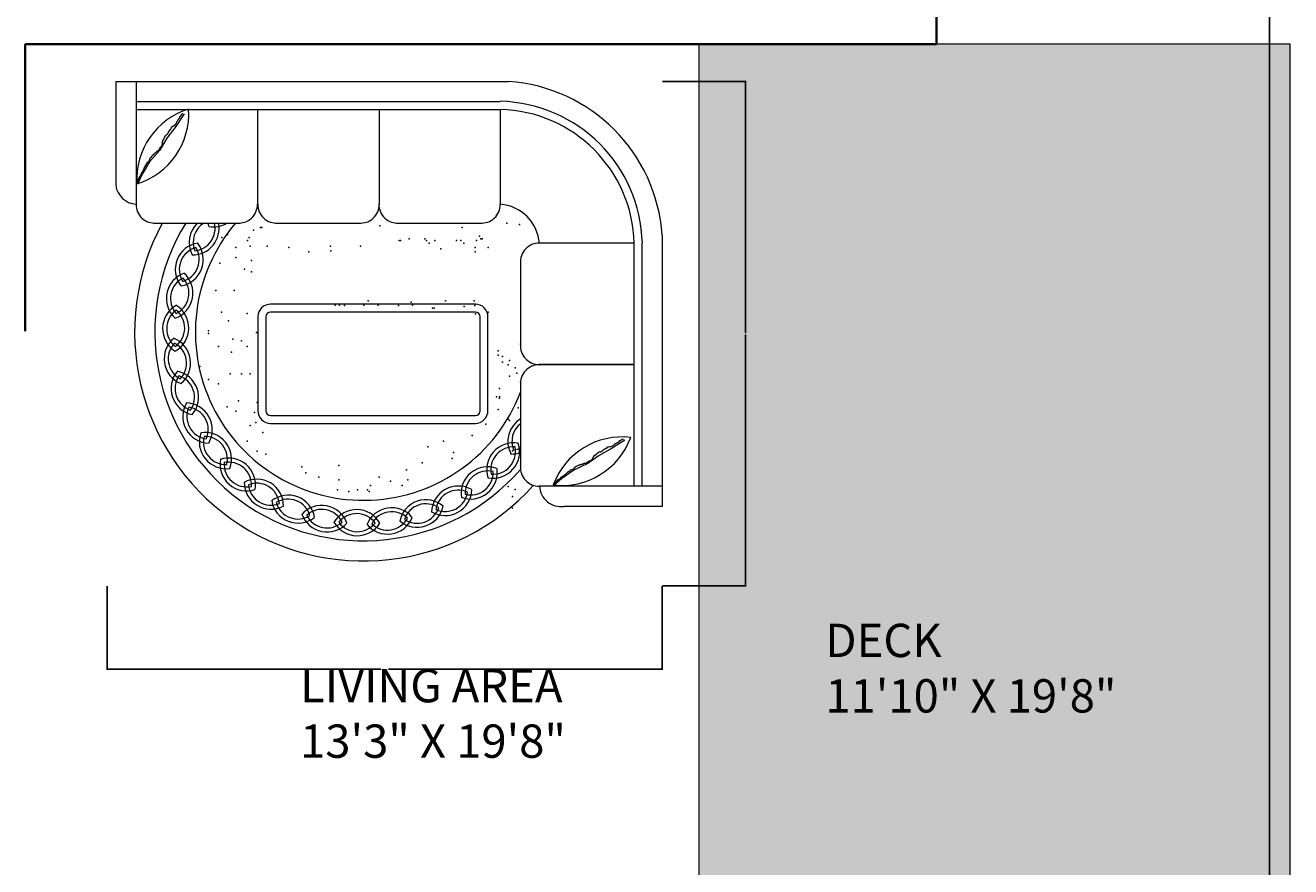
# Model space of a CAD drawing. Units: inches. Extents: x -4843 to -3402, y -164 to 3629.
# Tile 19 of 22: x -4303 to -3999, y 691 to 893. Entities that reach past the tile are written whole.
import ezdxf

# ---------------------------------------------------------------- set-up
doc = ezdxf.new("R2010")
doc.units = ezdxf.units.IN
for name, color, linetype, lineweight in [('A-ANNO-DIMS', 2, 'Continuous', 18), ('A-AREA-IDEN', 2, 'Continuous', 18), ('A-FLOR-DECK', 7, 'Continuous', 18), ('furniture', 6, 'Continuous', 18), ('walls', 7, 'Continuous', 35)]:
    doc.layers.add(name, color=color, linetype=linetype, lineweight=lineweight)
doc.layers.add('A-FLOR-PATT', color=30, linetype='Continuous', lineweight=13, true_color=0xf26722)
doc.styles.get("Standard").update_dxf_attribs({"font": 'arial.ttf'})
doc.dimstyles.get("Standard").update_dxf_attribs({"dimtxt": 0.18, "dimasz": 0.18, "dimexe": 0.18, "dimexo": 0.0625, "dimgap": 0.09, "dimtad": 0, "dimtih": 1, "dimtoh": 1, "dimdec": 4, "dimzin": 0, "dimdsep": 46, "dimtxsty": 'Standard', "dimcen": 0.09, "dimadec": 0, "dimazin": 0, "dimtfac": 1, "dimtdec": 4, "dimtofl": 0, "dimtmove": 0, "dimatfit": 3, "dimfxl": 1, "dimtolj": 1, "dimtzin": 0, "dimarcsym": 0})

# ---------------------------------------------------------------- blocks, each defined once
blk = doc.blocks.new('A$C2439112B')
for p, q in [((0, 2369.5), (1940.5, 2369.5)), ((0, 2369.5), (0, 1856.2)), ((100, 2369.5), (100, 1762.9)), ((1900, 2269.5), (100, 2269.5)), ((1900, 2229.5), (100, 2229.5)), ((338.3, 2209), (296.7, 2146.5)), ((317.5, 2195.1), (315.2, 2195.1)), ((315.2, 2195.1), (315.2, 2188.1)), ((318.7, 2196.2), (317.5, 2195.1)), ((319.8, 2198.5), (318.7, 2196.2)), ((322.1, 2199.7), (319.8, 2199.7)), ((319.8, 2199.7), (319.8, 2198.5)), ((324.5, 2204.3), (322.1, 2204.3)), ((322.1, 2204.3), (322.1, 2199.7)), ((326.8, 2206.6), (324.5, 2204.3)), ((327.9, 2209), (326.8, 2206.6)), ((331.4, 2209), (327.9, 2209)), ((700, 2229.5), (700, 1761.4)), ((1301.8, 2231.3), (1301.8, 1761.4)), ((1900, 2231.3), (1900, 1761.4)), ((296.7, 2146.5), (252.8, 2088.6)), ((265.5, 2129.1), (264.3, 2126.8)), ((264.3, 2126.8), (264.3, 2125.7)), ((267.8, 2129.1), (265.5, 2129.1)), ((270.1, 2133.7), (267.8, 2129.1)), ((271.3, 2133.7), (270.1, 2133.7)), ((273.6, 2143), (271.3, 2133.7)), ((275.9, 2143), (273.6, 2143)), ((277.1, 2144.2), (275.9, 2143)), ((279.4, 2145.3), (277.1, 2144.2)), ((280.5, 2147.6), (279.4, 2145.3)), ((285.1, 2147.6), (280.5, 2147.6)), ((286.3, 2149.9), (285.1, 2147.6)), ((287.5, 2149.9), (286.3, 2149.9)), ((292.1, 2152.3), (287.5, 2152.3)), ((287.5, 2152.3), (287.5, 2149.9)), ((293.2, 2156.9), (292.1, 2154.6)), ((292.1, 2154.6), (292.1, 2152.3)), ((294.4, 2156.9), (293.2, 2156.9)), ((295.6, 2158), (294.4, 2156.9)), ((296.7, 2160.4), (295.6, 2158)), ((299, 2161.5), (296.7, 2161.5)), ((296.7, 2161.5), (296.7, 2160.4)), ((300.2, 2169.6), (299, 2162.7)), ((299, 2162.7), (299, 2161.5)), ((301.3, 2169.6), (300.2, 2169.6)), ((303.6, 2170.8), (301.3, 2169.6)), ((304.8, 2177.7), (303.6, 2170.8)), ((308.3, 2177.7), (304.8, 2177.7)), ((310.6, 2182.3), (308.3, 2182.3)), ((308.3, 2182.3), (308.3, 2177.7)), ((311.7, 2184.7), (310.6, 2182.3)), ((312.9, 2185.8), (311.7, 2184.7)), ((314, 2187), (312.9, 2187)), ((312.9, 2187), (312.9, 2185.8)), ((315.2, 2188.1), (314, 2187)), ((252.8, 2088.6), (218.1, 2029.6)), ((229.6, 2064.3), (228.5, 2057.4)), ((230.8, 2073.6), (229.6, 2073.6)), ((229.6, 2073.6), (229.6, 2064.3)), ((232, 2074.7), (230.8, 2073.6)), ((233.1, 2081.7), (232, 2074.7)), ((235.4, 2081.7), (233.1, 2081.7)), ((236.6, 2082.8), (235.4, 2081.7)), ((237.7, 2089.8), (236.6, 2082.8)), ((238.9, 2089.8), (237.7, 2089.8)), ((240.1, 2090.9), (238.9, 2089.8)), ((241.2, 2097.9), (240.1, 2090.9)), ((243.5, 2097.9), (241.2, 2097.9)), ((245.8, 2102.5), (243.5, 2097.9)), ((247, 2102.5), (245.8, 2102.5)), ((248.1, 2103.7), (247, 2102.5)), ((250.5, 2104.8), (248.1, 2103.7)), ((251.6, 2107.1), (250.5, 2104.8)), ((252.8, 2107.1), (251.6, 2107.1)), ((255.1, 2109.5), (252.8, 2107.1)), ((256.2, 2111.8), (255.1, 2109.5)), ((257.4, 2111.8), (256.2, 2111.8)), ((259.7, 2118.7), (257.4, 2111.8)), ((260.9, 2119.9), (259.7, 2119.9)), ((259.7, 2119.9), (259.7, 2118.7)), ((262, 2122.2), (260.9, 2121)), ((260.9, 2121), (260.9, 2119.9)), ((263.2, 2124.5), (262, 2124.5)), ((262, 2124.5), (262, 2122.2)), ((264.3, 2125.7), (263.2, 2124.5)), ((218.1, 2029.6), (167.2, 1971.8)), ((179.9, 2003), (177.6, 2000.7)), ((182.2, 2005.3), (179.9, 2003)), ((184.6, 2005.3), (182.2, 2005.3)), ((186.9, 2007.6), (184.6, 2006.5)), ((184.6, 2006.5), (184.6, 2005.3)), ((190.3, 2010), (186.9, 2010)), ((186.9, 2010), (186.9, 2007.6)), ((191.5, 2012.3), (190.3, 2010)), ((193.8, 2014.6), (191.5, 2012.3)), ((195, 2014.6), (193.8, 2014.6)), ((201.9, 2021.5), (195, 2014.6)), ((204.2, 2022.7), (201.9, 2022.7)), ((201.9, 2022.7), (201.9, 2021.5)), ((205.4, 2023.8), (204.2, 2022.7)), ((206.5, 2025), (205.4, 2023.8)), ((207.7, 2027.3), (206.5, 2025)), ((211.2, 2027.3), (207.7, 2027.3)), ((212.3, 2034.2), (211.2, 2027.3)), ((213.5, 2035.4), (212.3, 2034.2)), ((215.8, 2035.4), (213.5, 2035.4)), ((218.1, 2042.3), (215.8, 2035.4)), ((220.4, 2043.5), (218.1, 2042.3)), ((222.7, 2045.8), (220.4, 2044.7)), ((220.4, 2044.7), (220.4, 2043.5)), ((223.9, 2048.1), (222.7, 2045.8)), ((226.2, 2048.1), (223.9, 2048.1)), ((227.3, 2055.1), (226.2, 2048.1)), ((228.5, 2057.4), (227.3, 2056.2)), ((227.3, 2056.2), (227.3, 2055.1)), ((167.2, 1971.8), (130.2, 1910.5)), ((139.5, 1938.2), (138.3, 1938.2)), ((138.3, 1938.2), (138.3, 1937.1)), ((140.6, 1945.2), (139.5, 1938.2)), ((141.8, 1946.3), (140.6, 1945.2)), ((142.9, 1946.3), (141.8, 1946.3)), ((145.2, 1950.9), (142.9, 1948.6)), ((142.9, 1948.6), (142.9, 1946.3)), ((147.6, 1954.4), (145.2, 1952.1)), ((145.2, 1952.1), (145.2, 1950.9)), ((149.9, 1956.7), (147.6, 1955.6)), ((147.6, 1955.6), (147.6, 1954.4)), ((151, 1963.7), (149.9, 1956.7)), ((152.2, 1963.7), (151, 1963.7)), ((154.5, 1966), (152.2, 1963.7)), ((155.7, 1968.3), (154.5, 1966)), ((156.8, 1968.3), (155.7, 1968.3)), ((159.1, 1970.6), (156.8, 1968.3)), ((160.3, 1972.9), (159.1, 1970.6)), ((161.4, 1972.9), (160.3, 1972.9)), ((162.6, 1974.1), (161.4, 1972.9)), ((163.7, 1976.4), (162.6, 1974.1)), ((166.1, 1977.6), (163.7, 1977.6)), ((163.7, 1977.6), (163.7, 1976.4)), ((168.4, 1986.8), (166.1, 1986.8)), ((166.1, 1986.8), (166.1, 1977.6)), ((169.5, 1991.4), (168.4, 1989.1)), ((168.4, 1989.1), (168.4, 1986.8)), ((170.7, 1991.4), (169.5, 1991.4)), ((173, 1993.8), (170.7, 1991.4)), ((174.2, 1996.1), (173, 1993.8)), ((177.6, 1999.5), (174.2, 1996.1)), ((177.6, 2000.7), (177.6, 1999.5)), ((130.2, 1910.5), (107.1, 1861.9)), ((109.4, 1878.1), (108.3, 1876.9)), ((108.3, 1876.9), (108.3, 1868.8)), ((110.6, 1878.1), (109.4, 1878.1)), ((112.9, 1886.2), (110.6, 1886.2)), ((110.6, 1886.2), (110.6, 1878.1)), ((114, 1894.3), (112.9, 1887.3)), ((112.9, 1887.3), (112.9, 1886.2)), ((115.2, 1895.4), (114, 1894.3)), ((116.3, 1898.9), (115.2, 1896.6)), ((115.2, 1896.6), (115.2, 1895.4)), ((117.5, 1898.9), (116.3, 1898.9)), ((118.7, 1900), (117.5, 1898.9)), ((119.8, 1902.4), (118.7, 1900)), ((122.1, 1903.5), (119.8, 1903.5)), ((119.8, 1903.5), (119.8, 1902.4)), ((123.3, 1912.8), (122.1, 1903.5)), ((125.6, 1912.8), (123.3, 1912.8)), ((127.9, 1917.4), (125.6, 1912.8)), ((129.1, 1917.4), (127.9, 1917.4)), ((131.4, 1922), (129.1, 1917.4)), ((132.5, 1922), (131.4, 1922)), ((133.7, 1929), (132.5, 1922)), ((134.8, 1930.1), (133.7, 1929)), ((136, 1930.1), (134.8, 1930.1)), ((138.3, 1937.1), (136, 1930.1)), ((107.1, 1866.5), (105.9, 1865.3)), ((108.3, 1868.8), (107.1, 1867.6)), ((107.1, 1867.6), (107.1, 1866.5)), ((185.7, 1669.5), (614.3, 1669.5)), ((787.6, 1669.5), (1201.8, 1669.5)), ((1385.7, 1669.5), (1800, 1669.5)), ((2561.5, 1570.5), (2093.3, 1570.5)), ((2560, 1570.5), (2560, 970.5)), ((2600, 1570.5), (2600, 970.5)), ((2700, 1610), (2700, 269.5)), ((2000, 1484.8), (2000, 1056.2)), ((1776.7, 1268.9), (765, 1268.9)), ((702.6, 1206.5), (702.6, 742.5)), ((741.6, 1206.5), (741.6, 742.5)), ((1776.7, 1229.9), (765, 1229.9)), ((1800.1, 742.5), (1800.1, 1206.5)), ((1839.1, 742.5), (1839.1, 1206.5)), ((2560, 970.5), (2091.8, 970.5)), ((2561.5, 969.5), (2093.3, 969.5)), ((2560, 969.5), (2560, 369.5)), ((2600, 969.5), (2600, 369.5)), ((2000, 883.8), (2000, 455.2)), ((765, 719.1), (1776.7, 719.1)), ((765, 680.1), (1776.7, 680.1)), ((2429.3, 563.4), (2423.5, 555.9)), ((2431.4, 562.5), (2429.3, 563.4)), ((2433, 563.1), (2431.4, 562.5)), ((2435.5, 563.2), (2433, 563.1)), ((2437.5, 564.8), (2435.5, 563.2)), ((2441.8, 563), (2437.5, 564.8)), ((2443.7, 564.6), (2441.8, 563)), ((2444.8, 564.2), (2443.7, 564.6)), ((2445.7, 566.3), (2444.8, 564.2)), ((2450, 564.4), (2445.7, 566.3)), ((2450.9, 566.5), (2450, 564.4)), ((2452.9, 568.2), (2450.9, 566.5)), ((2515.1, 597.7), (2451.9, 557.3)), ((2454, 567.7), (2452.9, 568.2)), ((2455.5, 568.3), (2454, 567.7)), ((2457.5, 570), (2455.5, 568.3)), ((2457.9, 571), (2457.5, 570)), ((2460, 570.1), (2457.9, 571)), ((2460.5, 571.2), (2460, 570.1)), ((2464.4, 577.1), (2460.5, 571.2)), ((2465.4, 576.6), (2464.4, 577.1)), ((2468, 576.7), (2465.4, 576.6)), ((2471.9, 582.6), (2468, 576.7)), ((2475, 581.2), (2471.9, 582.6)), ((2476.9, 585.4), (2475, 581.2)), ((2479, 584.5), (2476.9, 585.4)), ((2481, 586.2), (2479, 584.5)), ((2482.5, 586.8), (2481, 586.2)), ((2483, 587.8), (2482.5, 586.8)), ((2484.1, 587.4), (2483, 587.8)), ((2485.6, 588), (2484.1, 587.4)), ((2488.4, 594.3), (2485.6, 588)), ((2490.5, 593.4), (2488.4, 594.3)), ((2492, 594), (2490.5, 593.4)), ((2494, 595.6), (2492, 594)), ((2494.5, 596.7), (2494, 595.6)), ((2496.6, 595.7), (2494.5, 596.7)), ((2498.4, 600), (2496.6, 595.7)), ((2500.6, 599.1), (2498.4, 600)), ((2503.6, 600.2), (2500.6, 599.1)), ((2505.6, 601.9), (2503.6, 600.2)), ((2508.8, 600.5), (2505.6, 601.9)), ((2388.4, 522), (2332.9, 481.9)), ((2351.6, 501.5), (2347.7, 495.6)), ((2352.1, 502.6), (2351.6, 501.5)), ((2353.6, 503.2), (2352.1, 502.6)), ((2357.4, 509.1), (2353.6, 503.2)), ((2361.2, 517.5), (2357.4, 509.1)), ((2362.2, 517.1), (2361.2, 517.5)), ((2363.7, 517.7), (2362.2, 517.1)), ((2367.6, 523.6), (2363.7, 517.7)), ((2369.7, 522.6), (2367.6, 523.6)), ((2371.2, 523.2), (2369.7, 522.6)), ((2375.1, 529.1), (2371.2, 523.2)), ((2376.1, 528.6), (2375.1, 529.1)), ((2377.7, 529.2), (2376.1, 528.6)), ((2381.5, 535.1), (2377.7, 529.2)), ((2383.6, 534.2), (2381.5, 535.1)), ((2387.6, 537.5), (2383.6, 534.2)), ((2388.7, 537), (2387.6, 537.5)), ((2451.9, 557.3), (2388.4, 522)), ((2390.2, 537.6), (2388.7, 537)), ((2392.8, 537.8), (2390.2, 537.6)), ((2394.8, 539.4), (2392.8, 537.8)), ((2395.8, 538.9), (2394.8, 539.4)), ((2398.9, 540.1), (2395.8, 538.9)), ((2400.9, 541.8), (2398.9, 540.1)), ((2401.9, 541.3), (2400.9, 541.8)), ((2406.8, 546.7), (2401.9, 541.3)), ((2407.3, 547.8), (2406.8, 546.7)), ((2408.4, 547.3), (2407.3, 547.8)), ((2408.8, 548.4), (2408.4, 547.3)), ((2410.3, 549), (2408.8, 548.4)), ((2411.3, 551.1), (2410.3, 549)), ((2412.3, 550.6), (2411.3, 551.1)), ((2413.9, 551.2), (2412.3, 550.6)), ((2414.3, 552.3), (2413.9, 551.2)), ((2416.3, 553.9), (2414.3, 552.3)), ((2418.4, 553), (2416.3, 553.9)), ((2422.4, 556.3), (2418.4, 553)), ((2423.5, 555.9), (2422.4, 556.3)), ((2263, 449.5), (2204.5, 408.2)), ((2231.5, 438.1), (2230.5, 435.9)), ((2234.5, 439.2), (2231.5, 438.1)), ((2235, 440.3), (2234.5, 439.2)), ((2238, 441.5), (2235, 440.3)), ((2238.5, 442.5), (2238, 441.5)), ((2241.1, 442.7), (2238.5, 442.5)), ((2244.9, 448.6), (2241.1, 442.7)), ((2246, 448.1), (2244.9, 448.6)), ((2249, 449.3), (2246, 448.1)), ((2251, 450.9), (2249, 449.3)), ((2252.1, 450.5), (2251, 450.9)), ((2255.1, 451.7), (2252.1, 450.5)), ((2257.1, 453.3), (2255.1, 451.7)), ((2258.2, 452.8), (2257.1, 453.3)), ((2259.7, 453.4), (2258.2, 452.8)), ((2261.7, 455.1), (2259.7, 453.4)), ((2262.2, 456.2), (2261.7, 455.1)), ((2264.3, 455.2), (2262.2, 456.2)), ((2332.9, 481.9), (2263, 449.5)), ((2268, 463.7), (2264.3, 455.2)), ((2270.1, 462.8), (2268, 463.7)), ((2271.1, 464.9), (2270.1, 462.8)), ((2273.1, 466.5), (2271.1, 464.9)), ((2274.1, 466.1), (2273.1, 466.5)), ((2277.2, 467.3), (2274.1, 466.1)), ((2279.1, 468.9), (2277.2, 467.3)), ((2283.7, 470.7), (2279.1, 468.9)), ((2284.2, 471.8), (2283.7, 470.7)), ((2287.2, 472.9), (2284.2, 471.8)), ((2290.3, 474.1), (2287.2, 472.9)), ((2292.4, 473.2), (2290.3, 474.1)), ((2292.9, 474.3), (2292.4, 473.2)), ((2295.4, 474.4), (2292.9, 474.3)), ((2296.4, 476.5), (2295.4, 474.4)), ((2299.6, 475.1), (2296.4, 476.5)), ((2301.5, 476.8), (2299.6, 475.1)), ((2304.6, 477.9), (2301.5, 476.8)), ((2305.7, 477.5), (2304.6, 477.9)), ((2314.8, 481), (2305.7, 477.5)), ((2315.3, 482.1), (2314.8, 481)), ((2317.4, 481.2), (2315.3, 482.1)), ((2318.9, 481.8), (2317.4, 481.2)), ((2320.4, 482.4), (2318.9, 481.8)), ((2322.4, 484), (2320.4, 482.4)), ((2325.6, 482.6), (2322.4, 484)), ((2329.4, 488.5), (2325.6, 482.6)), ((2331, 489.1), (2329.4, 488.5)), ((2333.1, 488.2), (2331, 489.1)), ((2338, 493.6), (2333.1, 488.2)), ((2340.6, 493.7), (2338, 493.6)), ((2341, 494.8), (2340.6, 493.7)), ((2343.6, 494.9), (2341, 494.8)), ((2345.6, 496.6), (2343.6, 494.9)), ((2347.7, 495.6), (2345.6, 496.6)), ((2204.5, 408.2), (2163.7, 373)), ((2165.6, 377.3), (2164.1, 376.7)), ((2166.1, 378.3), (2165.6, 377.3)), ((2167.6, 378.9), (2166.1, 378.3)), ((2170.9, 386.3), (2167.6, 378.9)), ((2172.4, 386.9), (2170.9, 386.3)), ((2173.4, 386.5), (2172.4, 386.9)), ((2176.7, 393.9), (2173.4, 386.5)), ((2178.8, 393), (2176.7, 393.9)), ((2179.3, 394), (2178.8, 393)), ((2183.1, 399.9), (2179.3, 394)), ((2184.7, 400.5), (2183.1, 399.9)), ((2185.1, 401.6), (2184.7, 400.5)), ((2187.1, 403.2), (2185.1, 401.6)), ((2188.2, 402.7), (2187.1, 403.2)), ((2189.7, 403.3), (2188.2, 402.7)), ((2191.7, 405), (2189.7, 403.3)), ((2192.1, 406.1), (2191.7, 405)), ((2194.3, 405.1), (2192.1, 406.1)), ((2199.1, 413.1), (2194.3, 405.1)), ((2201.2, 412.2), (2199.1, 413.1)), ((2205.1, 415.5), (2201.2, 412.2)), ((2206.2, 415), (2205.1, 415.5)), ((2210.2, 418.3), (2206.2, 415)), ((2211.2, 417.9), (2210.2, 418.3)), ((2215.1, 423.8), (2211.2, 417.9)), ((2216.6, 424.4), (2215.1, 423.8)), ((2217.7, 423.9), (2216.6, 424.4)), ((2222.6, 429.3), (2217.7, 423.9)), ((2223.1, 430.4), (2222.6, 429.3)), ((2224.1, 429.9), (2223.1, 430.4)), ((2228, 435.8), (2224.1, 429.9)), ((2229.5, 436.4), (2228, 435.8)), ((2230.5, 435.9), (2229.5, 436.4)), ((2560, 369.5), (2091.8, 369.5)), ((2700, 369.5), (2093.3, 369.5)), ((2700, 269.5), (2215.3, 269.5))]:
    blk.add_line(p, q)
for centre, radius, start, end in [((1883.1, 1552.6), 818.9, 4.01764, 85.98236), ((1883.1, 1552.6), 718.9, 1.36318, 88.65199), ((465.7, 1886), 362.2, 106.97415, 183.5511), ((-1.5, 2210), 362.2, 286.97415, 3.5511), ((1883.1, 1552.6), 678.9, 1.44447, 88.57256), ((106.9, 1870.5), 107.9, 187.6347, 266.31517), ((192.9, 1762.1), 92.9, 179.5378, 274.41207), ((607.1, 1762.1), 92.9, 265.58793, 0.4622), ((794.7, 1762.1), 92.9, 179.5378, 274.41207), ((1209, 1762.1), 92.9, 265.58793, 0.4622), ((1392.9, 1762.1), 92.9, 179.5378, 274.41207), ((1807.1, 1762.1), 92.9, 265.58793, 0.4622), ((1883.1, 1552.6), 210.9, 4.59911, 85.40089), ((1224, 1130.5), 1130.7, 151.53032, 317.99926), ((1224, 1130.5), 1030.7, 148.47009, 318.86209), ((494.2, 1574.4), 131.9, 133.85137, 207.94088), ((378.9, 1644.1), 131.9, 269.72719, 11.09141), ((494.2, 1574.4), 111.9, 121.78467, 201.80816), ((378.9, 1644.1), 111.9, 275.8599, 13.10635), ((1224, 1130.5), 830.7, 139.54507, 339.09082), ((584.7, 1694.2), 131.9, 190.77752, 197.94088), ((483.3, 1782.9), 131.9, 259.72719, 300.7348), ((425.9, 1440.7), 131.9, 99.07785, 217.94088), ((300.3, 1489.4), 131.9, 279.72719, 38.59021), ((2092.6, 1477.6), 92.9, 89.5378, 184.41207), ((425.9, 1440.7), 111.9, 105.8599, 211.80816), ((300.3, 1489.4), 111.9, 285.8599, 31.80816), ((381.9, 1297.2), 131.9, 109.07785, 227.94088), ((381.9, 1297.2), 111.9, 115.8599, 221.80816), ((249.7, 1323.3), 131.9, 289.72719, 48.59021), ((249.7, 1323.3), 111.9, 295.8599, 41.80816), ((363.4, 1148.3), 131.9, 119.07785, 237.94088), ((228.7, 1151), 131.9, 299.72719, 58.59021), ((765, 1206.5), 62.4, 90, 180), ((1776.7, 1206.5), 62.4, 0, 90), ((363.4, 1148.3), 111.9, 125.8599, 231.80816), ((228.7, 1151), 111.9, 305.8599, 51.80816), ((765, 1206.5), 23.4, 90, 180), ((1776.7, 1206.5), 23.4, 0, 90), ((371.1, 998.4), 131.9, 129.07785, 247.94088), ((371.1, 998.4), 111.9, 135.8599, 241.80816), ((238, 977.7), 131.9, 309.72719, 68.59021), ((238, 977.7), 111.9, 315.8599, 61.80816), ((2092.6, 1063.3), 92.9, 175.58793, 270.4622), ((2092.6, 1063.3), 92.9, 175.58793, 270.4622), ((404.7, 852.1), 131.9, 139.07785, 257.94088), ((277.2, 808.6), 131.9, 319.72719, 78.59021), ((2092.6, 876.7), 92.9, 89.5378, 184.41207), ((404.7, 852.1), 111.9, 145.8599, 251.80816), ((277.2, 808.6), 111.9, 325.8599, 71.80816), ((463.2, 713.8), 131.9, 149.07785, 267.94088), ((345.2, 648.8), 131.9, 329.72719, 88.59021), ((463.2, 713.8), 111.9, 155.8599, 261.80816), ((345.2, 648.8), 111.9, 335.8599, 81.80816), ((765, 742.5), 62.4, 180, 270), ((765, 742.5), 23.4, 180, 270), ((1776.7, 742.5), 23.4, 270, 0), ((1776.7, 742.5), 62.4, 270, 0), ((2069.1, 590.4), 131.9, 121.59582, 208.59021), ((544.9, 587.9), 131.9, 159.07785, 277.94088), ((439.9, 503.4), 131.9, 339.72719, 98.59021), ((2069.1, 590.4), 111.9, 128.13878, 201.80816), ((544.9, 587.9), 111.9, 165.8599, 271.80816), ((439.9, 503.4), 111.9, 345.8599, 91.80816), ((1964.8, 451.7), 131.9, 79.72719, 198.59021), ((1863.3, 540.4), 131.9, 259.07785, 17.94088), ((1964.8, 451.7), 111.9, 85.8599, 191.80816), ((1863.3, 540.4), 111.9, 265.8599, 11.80816), ((2501.7, 250.8), 362.2, 83.23923, 159.81618), ((2204.5, 735.4), 362.2, 263.23923, 339.81618), ((647.1, 478), 131.9, 169.07785, 287.94088), ((558.4, 376.5), 131.9, 349.72719, 108.59021), ((1953.8, 660.2), 131.9, 269.07785, 290.50822), ((1953.8, 660.2), 111.9, 275.8599, 294.39097), ((647.1, 478), 111.9, 175.8599, 281.80816), ((558.4, 376.5), 111.9, 355.8599, 101.80816), ((1837.9, 333.2), 131.9, 69.72719, 188.59021), ((1753.4, 438.1), 131.9, 249.07785, 7.94088), ((1837.9, 333.2), 111.9, 75.8599, 181.80816), ((1753.4, 438.1), 111.9, 255.8599, 1.80816), ((2092.6, 462.4), 92.9, 175.58793, 270.4622), ((2092.6, 462.4), 92.9, 175.58793, 270.4622), ((697.1, 272.2), 131.9, 359.72719, 118.59021), ((766.9, 387.5), 131.9, 179.07785, 297.94088), ((697.1, 272.2), 111.9, 5.8599, 111.80816), ((766.9, 387.5), 111.9, 185.8599, 291.80816), ((851.9, 193.5), 131.9, 9.72719, 128.59021), ((1627.5, 356.5), 131.9, 239.07785, 357.94088), ((1692.5, 238.5), 131.9, 59.72719, 178.59021), ((1692.5, 238.5), 111.9, 65.8599, 171.80816), ((1627.5, 356.5), 111.9, 245.8599, 351.80816), ((2201, 376.5), 107.9, 183.68483, 277.6347), ((900.6, 319.2), 131.9, 189.07785, 307.94088), ((851.9, 193.5), 111.9, 15.8599, 121.80816), ((900.6, 319.2), 111.9, 195.8599, 301.80816), ((1018, 143), 131.9, 19.72719, 138.59021), ((1018, 143), 111.9, 25.8599, 131.80816), ((1190.3, 122), 131.9, 29.72719, 148.59021), ((1363.6, 131.2), 131.9, 39.72719, 158.59021), ((1489.2, 298), 131.9, 229.07785, 347.94088), ((1532.7, 170.5), 131.9, 49.72719, 168.59021), ((1532.7, 170.5), 111.9, 55.8599, 161.80816), ((1489.2, 298), 111.9, 235.8599, 341.80816), ((1044.1, 275.2), 131.9, 199.07785, 317.94088), ((1044.1, 275.2), 111.9, 205.8599, 311.80816), ((1193, 256.7), 131.9, 209.07785, 327.94088), ((1190.3, 122), 111.9, 35.8599, 141.80816), ((1193, 256.7), 111.9, 215.8599, 321.80816), ((1342.9, 264.4), 131.9, 219.07785, 337.94088), ((1363.6, 131.2), 111.9, 45.8599, 151.80816), ((1342.9, 264.4), 111.9, 225.8599, 331.80816)]:
    blk.add_arc(centre, radius, start, end)
for p in [(679.9, 1633.9), (715.3, 1648.1), (722.4, 1648.1), (1305, 1655.2), (1711.9, 1648.1), (1931.5, 1669.3), (1995.2, 1662.3), (524, 1598.5), (552.4, 1612.6), (651.5, 1584.3), (658.6, 1598.5), (1400.3, 1584.3), (1407.4, 1584.3), (1449.9, 1591.4), (1527.8, 1591.4), (1534.9, 1584.3), (1549, 1570.1), (1577.3, 1584.3), (1683.6, 1584.3), (1704.8, 1584.3), (1719, 1570.1), (1782.7, 1584.3), (1796.9, 1605.6), (1804, 1591.4), (1811.1, 1591.4), (592.8, 1548.9), (663.7, 1555.9), (748.7, 1555.9), (854.9, 1548.9), (954.1, 1527.6), (954.1, 1527.6), (1060.3, 1555.9), (1062.9, 1532.3), (1209, 1555.9), (1605.7, 1541.8), (1775.7, 1548.9), (1775.7, 1527.6), (1839.4, 1548.9), (514.9, 1470.9), (592.8, 1499.2), (635.3, 1442.5), (670.7, 1485.1), (670.7, 1428.4), (493.7, 1336.2), (585.8, 1336.2), (1084.1, 1264.2), (1105.4, 1264.2), (1129.4, 1262.8), (1225.8, 1264.2), (1247, 1285.5), (1296.6, 1264.2), (1396.5, 1262.8), (1459.5, 1278.4), (1466.6, 1264.2), (1629.5, 1285.5), (1721.6, 1257.1), (1771.2, 1285.5), (1774, 1262.8), (522, 1229.9), (649.5, 1222.8), (1565.8, 1250), (1572.8, 1250), (1778.2, 1221.7), (1840.3, 1229.3), (458.3, 1137.8), (557.4, 1187.4), (694.6, 1129.5), (458.3, 1123.6), (578.7, 1095.2), (621.2, 1088.2), (2000, 1070.5), (507.8, 1059.8), (571.6, 1031.4), (649.5, 1059.8), (1889, 1038.5), (1889, 1017.3), (1910.2, 1010.2), (415.8, 960.6), (1910.2, 981.8), (1938.6, 968.6), (1945.7, 991.4), (1974, 954.4), (2093.3, 969.5), (458.3, 896.8), (507.8, 875.5), (564.5, 925.1), (621.2, 925.1), (663.7, 925.1), (1945.7, 913.4), (1981.1, 927.6), (2000, 883.8), (1895.8, 851.9), (383.9, 774.9), (550.3, 762.1), (607, 790.5), (699.1, 783.4), (1881.9, 811.7), (1896.1, 811.7), (1896.1, 804.6), (1988.1, 757.5), (592.8, 740.9), (684.9, 733.8), (1889, 747.9), (1938.6, 700.8), (1945.7, 693.7), (663.7, 670), (692, 684.2), (727.4, 634.5), (1827.8, 675.9), (649.5, 592), (1541.9, 563.7), (1619.8, 592), (1761.5, 620.4), (699.1, 542.4), (741.6, 528.2), (1662.3, 507), (1669.4, 535.3), (1952.7, 530.7), (1959.8, 544.9), (918.6, 464.4), (1102.8, 471.5), (1435.7, 450.3), (1513.6, 485.7), (2000, 469.5), (939.9, 436.1), (1003.6, 414.8), (1102.8, 400.6), (1301.1, 414.8), (1357.8, 393.6), (1442.8, 400.6), (1095.7, 351), (1152.4, 343.9), (1194.9, 351), (1244.5, 351), (1251.5, 343.9), (1258.6, 372.3), (1414.4, 372.3), (1938.6, 367.7), (1959.8, 318), (1974, 353.5), (1959.8, 261.3)]:
    blk.add_point(p)
blk = doc.blocks.new('*D54')
at = {"layer": 'A-ANNO-DIMS', "color": 0, "lineweight": -2, "transparency": 16777216}
for p, q in [((-4283.13, 758.02), (-4283.13, 737.89)), ((-4149.69, 758.02), (-4149.69, 737.89)), ((-4282.95, 738.07), (-4217.35, 738.07)), ((-4149.87, 738.07), (-4215.46, 738.07))]:
    blk.add_line(p, q, dxfattribs=at)
at = {"layer": 'A-ANNO-DIMS', "color": 0, "transparency": 16777216}
for points in [[(-4282.95, 738.1), (-4282.95, 738.04), (-4283.13, 738.07)], [(-4149.87, 738.1), (-4149.87, 738.04), (-4149.69, 738.07)]]:
    blk.add_solid(points, dxfattribs=at)
at = {"layer": 'Defpoints', "color": 0, "transparency": 16777216}
for p in [(-4283.13, 758.08), (-4149.69, 758.08), (-4149.69, 738.07)]:
    blk.add_point(p, dxfattribs=at)
at = {"layer": 'A-ANNO-DIMS', "color": 0, "transparency": 16777216, "insert": (-4216.41, 738.07), "char_height": 0.18, "attachment_point": 5}
blk.add_mtext('\\A1;SOFA SET 133', dxfattribs=at)
blk = doc.blocks.new('*D55')
at = {"layer": 'A-ANNO-DIMS', "color": 0, "lineweight": -2, "transparency": 16777216}
for p, q in [((-4149.62, 879.37), (-4129.49, 879.37)), ((-4129.67, 879.19), (-4129.67, 818.91)), ((-4129.67, 758.26), (-4129.67, 818.54)), ((-4149.62, 758.08), (-4129.49, 758.08))]:
    blk.add_line(p, q, dxfattribs=at)
at = {"layer": 'A-ANNO-DIMS', "color": 0, "transparency": 16777216}
for points in [[(-4129.7, 879.19), (-4129.64, 879.19), (-4129.67, 879.37)], [(-4129.7, 758.26), (-4129.64, 758.26), (-4129.67, 758.08)]]:
    blk.add_solid(points, dxfattribs=at)
at = {"layer": 'Defpoints', "color": 0, "transparency": 16777216}
for p in [(-4149.69, 879.37), (-4129.67, 879.37), (-4149.69, 758.08)]:
    blk.add_point(p, dxfattribs=at)
at = {"layer": 'A-ANNO-DIMS', "color": 0, "transparency": 16777216, "insert": (-4129.67, 818.72), "char_height": 0.18, "attachment_point": 5}
blk.add_mtext('\\A1;121', dxfattribs=at)
blk = doc.blocks.new('*D81')
at = {"layer": 'A-ANNO-DIMS', "color": 0, "lineweight": -2, "transparency": 16777216}
for p, q in [((-4332.78, 86.42), (-4332.78, 1392.95)), ((-4332.6, 1392.77), (-4168.61, 1392.77)), ((-4003.86, 1392.77), (-4167.86, 1392.77)), ((-4003.68, 86.42), (-4003.68, 1392.95))]:
    blk.add_line(p, q, dxfattribs=at)
at = {"layer": 'A-ANNO-DIMS', "color": 0, "transparency": 16777216}
for points in [[(-4332.6, 1392.8), (-4332.6, 1392.74), (-4332.78, 1392.77)], [(-4003.86, 1392.8), (-4003.86, 1392.74), (-4003.68, 1392.77)]]:
    blk.add_solid(points, dxfattribs=at)
at = {"layer": 'Defpoints', "color": 0, "transparency": 16777216}
for p in [(-4003.68, 1392.77), (-4332.78, 86.35), (-4003.68, 86.35)]:
    blk.add_point(p, dxfattribs=at)
at = {"layer": 'A-ANNO-DIMS', "color": 0, "transparency": 16777216, "insert": (-4168.23, 1392.77), "char_height": 0.18, "attachment_point": 5}
blk.add_mtext('\\A1;329.1', dxfattribs=at)

msp = doc.modelspace()

# ---------------------------------------------------------------- hatches: boundary and pattern name
at = {"layer": 'A-FLOR-PATT', "transparency": 33554472}
h = msp.add_hatch(color=256, dxfattribs=at)
h.dxf.hatch_style = 1
h.paths.add_polyline_path([(-4538.62, 643.09), (-4595.62, 643.09), (-4666.62, 643.09), (-4666.62, 466.09), (-4595.62, 466.09), (-4538.62, 466.09)])
h.paths.add_polyline_path([(-3998.62, 888.09), (-4083.62, 888.09), (-4140.62, 888.09), (-4140.62, 652.09), (-4132.62, 652.09), (-4132.62, 650.09), (-4096.62, 650.09), (-4096.62, 652.09), (-4083.62, 652.09), (-3998.62, 652.09)])

# ---------------------------------------------------------------- linework, layer by layer
at = {"layer": 'A-FLOR-DECK'}
for p, q in [((-4140.78, 652.35), (-4140.78, 888.35)), ((-3998.78, 888.35), (-4083.78, 888.35)), ((-3998.78, 652.35), (-3998.78, 888.35))]:
    msp.add_line(p, q, dxfattribs=at)
at = {"layer": 'walls'}
for p, q in [((-4083.78, 1020.35), (-4083.78, 888.35)), ((-4302.78, 888.35), (-4083.78, 888.35)), ((-4302.78, 888.35), (-4302.78, 819.35))]:
    msp.add_line(p, q, dxfattribs=at)

# ---------------------------------------------------------------- block references
at = {"layer": 'furniture', "xscale": 0.048648506631742, "yscale": 0.048648506631742, "zscale": 0.048648506631742}
msp.add_blockref('A$C2439112B', (-4281.04, 764.09), dxfattribs=at)

# ---------------------------------------------------------------- texts
at = {"layer": 'A-AREA-IDEN', "char_height": 8, "attachment_point": 1}
for s, width, insert in [('DECK \\P11\'10" X 19\'8"', 80.3724, (-4110.47, 749)), ('LIVING AREA\\P13\'3" X 19\'8"', 78.1267, (-4236.73, 738.12))]:
    msp.add_mtext_dynamic_manual_height_columns(s, width=width, gutter_width=60, heights=[0], dxfattribs=dict(at, insert=insert))

# ---------------------------------------------------------------- dimensions: what is measured, and where the dimension line sits
at = {"layer": 'A-ANNO-DIMS'}
dim = msp.add_linear_dim(base=(-4003.68, 1392.77), p1=(-4332.78, 86.35), p2=(-4003.68, 86.35), dimstyle='Standard', override={"dimdec": 1, "dimlfac": 1, "dimrnd": 0, "dimzin": 0, "dimdsep": 46, "dimlunit": 2}, dxfattribs=at)
dim.commit()
dim.dimension.update_dxf_attribs({"geometry": '*D81', "text_midpoint": (-4168.23, 1392.77)})
dim = msp.add_linear_dim(base=(-4129.67, 879.37), p1=(-4149.69, 758.08), p2=(-4149.69, 879.37), angle=90, dimstyle='Standard', override={"dimdec": 0, "dimlfac": 1, "dimrnd": 0, "dimzin": 0, "dimdsep": 46, "dimlunit": 2}, dxfattribs=at)
dim.commit()
dim.dimension.update_dxf_attribs({"geometry": '*D55', "text_midpoint": (-4129.67, 818.72)})
dim = msp.add_linear_dim(base=(-4149.69, 738.07), p1=(-4283.13, 758.08), p2=(-4149.69, 758.08), text='SOFA SET <>', dimstyle='Standard', override={"dimdec": 0, "dimlfac": 1, "dimrnd": 0, "dimzin": 0, "dimdsep": 46, "dimlunit": 2}, dxfattribs=at)
dim.commit()
dim.dimension.update_dxf_attribs({"geometry": '*D54', "text_midpoint": (-4216.41, 738.07)})

doc.saveas('drawing.dxf')
